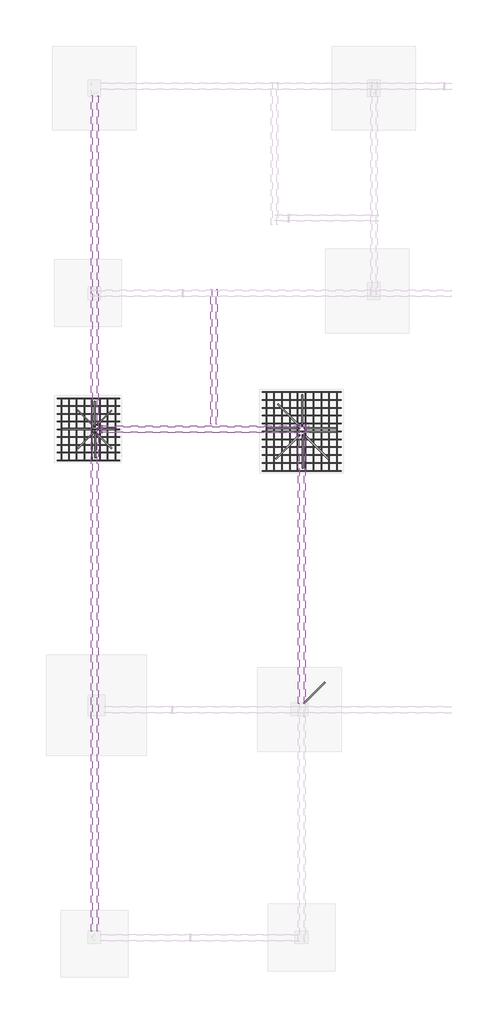
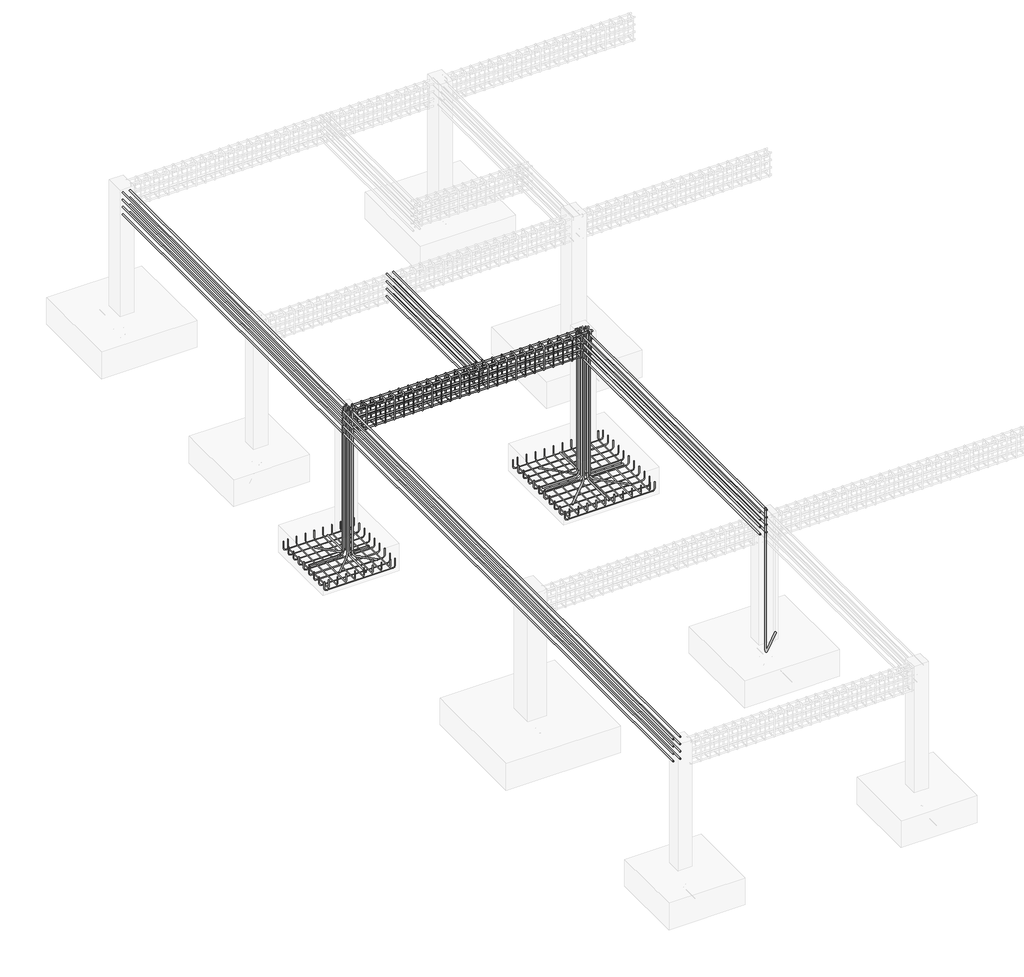
# One storey, part 5 of 10: 33 reinforcing bars.
"""IFC4 building model written with IfcOpenShell, lengths in millimetres."""

from ifc_helpers import new_model, si_unit, point, frame, origin, place, context, project, spatial, polyline, circle_curve, trimmed, segment, composite_curve, source, transform, mapped, element, save
from ifc_brep_helpers import swept_disk

model = new_model("IFC4")

# Units and contexts
model_context = context("Model", 3, world=origin())
ifc_project = project(units=[si_unit("LENGTHUNIT", "METRE", prefix="MILLI")], contexts=[model_context])

# Site, building, storey
site = spatial("IfcSite", under=ifc_project)
building = spatial("IfcBuilding", under=site)
storey = spatial("IfcBuildingStorey", under=building, Elevation=-2133.6)

# Reinforcing bars
placement = place(None, origin())
reinforcing_bar_shape = source(origin(), model_context, "Body", "SolidModel", [
    swept_disk(composite_curve([segment(polyline([(-4484.7164362, 6505.3219177, -2393.6), (-4484.7164362, 6505.3219177, -2504.1)]), True, "CONTINUOUS"), segment(trimmed(circle_curve(frame((-4519.4664362, 6505.3219177, -2504.1), z_axis=(0.0, 1.0, 0.0), x_axis=(34.75, 0.0, 0.0)), 34.75), [point((-4484.7164362, 6505.3219177, -2504.1))], [point((-4519.4664362, 6505.3219177, -2538.85))], True, "CARTESIAN"), True, "CONTINUOUS"), segment(polyline([(-4519.4664362, 6505.3219177, -2538.85), (-5579.6664362, 6505.3219177, -2538.85)]), True, "CONTINUOUS"), segment(trimmed(circle_curve(frame((-5579.6664362, 6505.3219177, -2504.1), z_axis=(0.0, 1.0, 0.0), x_axis=(0.0, 0.0, -34.75)), 34.75), [point((-5579.6664362, 6505.3219177, -2538.85))], [point((-5614.4164362, 6505.3219177, -2504.1))], True, "CARTESIAN"), True, "CONTINUOUS"), segment(polyline([(-5614.4164362, 6505.3219177, -2504.1), (-5614.4164362, 6505.3219177, -2393.6)]), True, "CONTINUOUS")], self_intersect=False), 4.75),
])
element("IfcReinforcingBar", 1, at=placement, inside=storey, context=model_context, shape_type="MappedRepresentation", body=[
    mapped(reinforcing_bar_shape, transform((0.0, 0.0, 0.0), x_axis=(1.0, 0.0, 0.0), y_axis=(0.0, 1.0, 0.0), z_axis=(0.0, 0.0, 1.0))),
    mapped(reinforcing_bar_shape, transform((0.0, -141.2125, 0.0), x_axis=(1.0, 0.0, 0.0), y_axis=(0.0, 1.0, 0.0), z_axis=(0.0, 0.0, 1.0))),
    mapped(reinforcing_bar_shape, transform((0.0, -282.425, 0.0), x_axis=(1.0, 0.0, 0.0), y_axis=(0.0, 1.0, 0.0), z_axis=(0.0, 0.0, 1.0))),
    mapped(reinforcing_bar_shape, transform((0.0, -423.6375, 0.0), x_axis=(1.0, 0.0, 0.0), y_axis=(0.0, 1.0, 0.0), z_axis=(0.0, 0.0, 1.0))),
    mapped(reinforcing_bar_shape, transform((0.0, -564.85, 0.0), x_axis=(1.0, 0.0, 0.0), y_axis=(0.0, 1.0, 0.0), z_axis=(0.0, 0.0, 1.0))),
    mapped(reinforcing_bar_shape, transform((0.0, -706.0625, 0.0), x_axis=(1.0, 0.0, 0.0), y_axis=(0.0, 1.0, 0.0), z_axis=(0.0, 0.0, 1.0))),
    mapped(reinforcing_bar_shape, transform((0.0, -847.275, 0.0), x_axis=(1.0, 0.0, 0.0), y_axis=(0.0, 1.0, 0.0), z_axis=(0.0, 0.0, 1.0))),
    mapped(reinforcing_bar_shape, transform((0.0, -988.4875, 0.0), x_axis=(1.0, 0.0, 0.0), y_axis=(0.0, 1.0, 0.0), z_axis=(0.0, 0.0, 1.0))),
    mapped(reinforcing_bar_shape, transform((0.0, -1129.7, 0.0), x_axis=(1.0, 0.0, 0.0), y_axis=(0.0, 1.0, 0.0), z_axis=(0.0, 0.0, 1.0))),
])
reinforcing_bar_2_shape = source(origin(), model_context, "Body", "SolidModel", [
    swept_disk(composite_curve([segment(polyline([(-4559.6743867, 5375.6219177, -2379.223371), (-4559.6743867, 5375.6219177, -2489.723371)]), True, "CONTINUOUS"), segment(trimmed(circle_curve(frame((-4559.6743867, 5410.3719177, -2489.723371), z_axis=(1.0, 0.0, 0.0), x_axis=(0.0, -34.75, 0.0)), 34.75), [point((-4559.6743867, 5375.6219177, -2489.723371))], [point((-4559.6743867, 5410.3719177, -2524.473371))], True, "CARTESIAN"), True, "CONTINUOUS"), segment(polyline([(-4559.6743867, 5410.3719177, -2524.473371), (-4559.6743867, 6470.5719177, -2524.473371)]), True, "CONTINUOUS"), segment(trimmed(circle_curve(frame((-4559.6743867, 6470.5719177, -2489.723371), z_axis=(1.0, 0.0, 0.0), x_axis=(0.0, 0.0, -34.75)), 34.75), [point((-4559.6743867, 6470.5719177, -2524.473371))], [point((-4559.6743867, 6505.3219177, -2489.723371))], True, "CARTESIAN"), True, "CONTINUOUS"), segment(polyline([(-4559.6743867, 6505.3219177, -2489.723371), (-4559.6743867, 6505.3219177, -2379.223371)]), True, "CONTINUOUS")], self_intersect=False), 4.75),
])
element("IfcReinforcingBar", 2, at=placement, inside=storey, context=model_context, shape_type="MappedRepresentation", body=[
    mapped(reinforcing_bar_2_shape, transform((0.0, 0.0, 0.0), x_axis=(1.0, 0.0, 0.0), y_axis=(0.0, 1.0, 0.0), z_axis=(0.0, 0.0, 1.0))),
    mapped(reinforcing_bar_2_shape, transform((-140.5079612, 0.0, 0.0), x_axis=(1.0, 0.0, 0.0), y_axis=(0.0, 1.0, 0.0), z_axis=(0.0, 0.0, 1.0))),
    mapped(reinforcing_bar_2_shape, transform((-281.0159224, 0.0, 0.0), x_axis=(1.0, 0.0, 0.0), y_axis=(0.0, 1.0, 0.0), z_axis=(0.0, 0.0, 1.0))),
    mapped(reinforcing_bar_2_shape, transform((-421.5238836, 0.0, 0.0), x_axis=(1.0, 0.0, 0.0), y_axis=(0.0, 1.0, 0.0), z_axis=(0.0, 0.0, 1.0))),
    mapped(reinforcing_bar_2_shape, transform((-562.0318448, 0.0, 0.0), x_axis=(1.0, 0.0, 0.0), y_axis=(0.0, 1.0, 0.0), z_axis=(0.0, 0.0, 1.0))),
    mapped(reinforcing_bar_2_shape, transform((-702.539806, 0.0, 0.0), x_axis=(1.0, 0.0, 0.0), y_axis=(0.0, 1.0, 0.0), z_axis=(0.0, 0.0, 1.0))),
    mapped(reinforcing_bar_2_shape, transform((-843.0477672, 0.0, 0.0), x_axis=(1.0, 0.0, 0.0), y_axis=(0.0, 1.0, 0.0), z_axis=(0.0, 0.0, 1.0))),
    mapped(reinforcing_bar_2_shape, transform((-983.5557284, 0.0, 0.0), x_axis=(1.0, 0.0, 0.0), y_axis=(0.0, 1.0, 0.0), z_axis=(0.0, 0.0, 1.0))),
])
reinforcing_bar_3_shape = source(origin(), model_context, "Body", "SolidModel", [
    swept_disk(composite_curve([segment(polyline([(-446.1164362, 6619.6219177, -2393.6), (-446.1164362, 6619.6219177, -2504.1)]), True, "CONTINUOUS"), segment(trimmed(circle_curve(frame((-480.8664362, 6619.6219177, -2504.1), z_axis=(0.0, 1.0, 0.0), x_axis=(34.75, 0.0, 0.0)), 34.75), [point((-446.1164362, 6619.6219177, -2504.1))], [point((-480.8664362, 6619.6219177, -2538.85))], True, "CARTESIAN"), True, "CONTINUOUS"), segment(polyline([(-480.8664362, 6619.6219177, -2538.85), (-1845.8664362, 6619.6219177, -2538.85)]), True, "CONTINUOUS"), segment(trimmed(circle_curve(frame((-1845.8664362, 6619.6219177, -2504.1), z_axis=(0.0, 1.0, 0.0), x_axis=(0.0, 0.0, -34.75)), 34.75), [point((-1845.8664362, 6619.6219177, -2538.85))], [point((-1880.6164362, 6619.6219177, -2504.1))], True, "CARTESIAN"), True, "CONTINUOUS"), segment(polyline([(-1880.6164362, 6619.6219177, -2504.1), (-1880.6164362, 6619.6219177, -2393.6)]), True, "CONTINUOUS")], self_intersect=False), 4.75),
])
element("IfcReinforcingBar", 3, at=placement, inside=storey, context=model_context, shape_type="MappedRepresentation", body=[
    mapped(reinforcing_bar_3_shape, transform((0.0, 0.0, 0.0), x_axis=(1.0, 0.0, 0.0), y_axis=(0.0, 1.0, 0.0), z_axis=(0.0, 0.0, 1.0))),
    mapped(reinforcing_bar_3_shape, transform((0.0, -143.45, 0.0), x_axis=(1.0, 0.0, 0.0), y_axis=(0.0, 1.0, 0.0), z_axis=(0.0, 0.0, 1.0))),
    mapped(reinforcing_bar_3_shape, transform((0.0, -286.9, 0.0), x_axis=(1.0, 0.0, 0.0), y_axis=(0.0, 1.0, 0.0), z_axis=(0.0, 0.0, 1.0))),
    mapped(reinforcing_bar_3_shape, transform((0.0, -430.35, 0.0), x_axis=(1.0, 0.0, 0.0), y_axis=(0.0, 1.0, 0.0), z_axis=(0.0, 0.0, 1.0))),
    mapped(reinforcing_bar_3_shape, transform((0.0, -573.8, 0.0), x_axis=(1.0, 0.0, 0.0), y_axis=(0.0, 1.0, 0.0), z_axis=(0.0, 0.0, 1.0))),
    mapped(reinforcing_bar_3_shape, transform((0.0, -717.25, 0.0), x_axis=(1.0, 0.0, 0.0), y_axis=(0.0, 1.0, 0.0), z_axis=(0.0, 0.0, 1.0))),
    mapped(reinforcing_bar_3_shape, transform((0.0, -860.7, 0.0), x_axis=(1.0, 0.0, 0.0), y_axis=(0.0, 1.0, 0.0), z_axis=(0.0, 0.0, 1.0))),
    mapped(reinforcing_bar_3_shape, transform((0.0, -1004.15, 0.0), x_axis=(1.0, 0.0, 0.0), y_axis=(0.0, 1.0, 0.0), z_axis=(0.0, 0.0, 1.0))),
    mapped(reinforcing_bar_3_shape, transform((0.0, -1147.6, 0.0), x_axis=(1.0, 0.0, 0.0), y_axis=(0.0, 1.0, 0.0), z_axis=(0.0, 0.0, 1.0))),
    mapped(reinforcing_bar_3_shape, transform((0.0, -1291.05, 0.0), x_axis=(1.0, 0.0, 0.0), y_axis=(0.0, 1.0, 0.0), z_axis=(0.0, 0.0, 1.0))),
    mapped(reinforcing_bar_3_shape, transform((0.0, -1434.5, 0.0), x_axis=(1.0, 0.0, 0.0), y_axis=(0.0, 1.0, 0.0), z_axis=(0.0, 0.0, 1.0))),
])
reinforcing_bar_4_shape = source(origin(), model_context, "Body", "SolidModel", [
    swept_disk(composite_curve([segment(polyline([(-521.0743867, 5185.1219177, -2379.223371), (-521.0743867, 5185.1219177, -2489.723371)]), True, "CONTINUOUS"), segment(trimmed(circle_curve(frame((-521.0743867, 5219.8719177, -2489.723371), z_axis=(1.0, 0.0, 0.0), x_axis=(0.0, -34.75, 0.0)), 34.75), [point((-521.0743867, 5185.1219177, -2489.723371))], [point((-521.0743867, 5219.8719177, -2524.473371))], True, "CARTESIAN"), True, "CONTINUOUS"), segment(polyline([(-521.0743867, 5219.8719177, -2524.473371), (-521.0743867, 6584.8719177, -2524.473371)]), True, "CONTINUOUS"), segment(trimmed(circle_curve(frame((-521.0743867, 6584.8719177, -2489.723371), z_axis=(1.0, 0.0, 0.0), x_axis=(0.0, 0.0, -34.75)), 34.75), [point((-521.0743867, 6584.8719177, -2524.473371))], [point((-521.0743867, 6619.6219177, -2489.723371))], True, "CARTESIAN"), True, "CONTINUOUS"), segment(polyline([(-521.0743867, 6619.6219177, -2489.723371), (-521.0743867, 6619.6219177, -2379.223371)]), True, "CONTINUOUS")], self_intersect=False), 4.75),
])
element("IfcReinforcingBar", 4, at=placement, inside=storey, context=model_context, shape_type="MappedRepresentation", body=[
    mapped(reinforcing_bar_4_shape, transform((0.0, 0.0, 0.0), x_axis=(1.0, 0.0, 0.0), y_axis=(0.0, 1.0, 0.0), z_axis=(0.0, 0.0, 1.0))),
    mapped(reinforcing_bar_4_shape, transform((-143.1506365, 0.0, 0.0), x_axis=(1.0, 0.0, 0.0), y_axis=(0.0, 1.0, 0.0), z_axis=(0.0, 0.0, 1.0))),
    mapped(reinforcing_bar_4_shape, transform((-286.301273, 0.0, 0.0), x_axis=(1.0, 0.0, 0.0), y_axis=(0.0, 1.0, 0.0), z_axis=(0.0, 0.0, 1.0))),
    mapped(reinforcing_bar_4_shape, transform((-429.4519095, 0.0, 0.0), x_axis=(1.0, 0.0, 0.0), y_axis=(0.0, 1.0, 0.0), z_axis=(0.0, 0.0, 1.0))),
    mapped(reinforcing_bar_4_shape, transform((-572.602546, 0.0, 0.0), x_axis=(1.0, 0.0, 0.0), y_axis=(0.0, 1.0, 0.0), z_axis=(0.0, 0.0, 1.0))),
    mapped(reinforcing_bar_4_shape, transform((-715.7531825, 0.0, 0.0), x_axis=(1.0, 0.0, 0.0), y_axis=(0.0, 1.0, 0.0), z_axis=(0.0, 0.0, 1.0))),
    mapped(reinforcing_bar_4_shape, transform((-858.903819, 0.0, 0.0), x_axis=(1.0, 0.0, 0.0), y_axis=(0.0, 1.0, 0.0), z_axis=(0.0, 0.0, 1.0))),
    mapped(reinforcing_bar_4_shape, transform((-1002.0544555, 0.0, 0.0), x_axis=(1.0, 0.0, 0.0), y_axis=(0.0, 1.0, 0.0), z_axis=(0.0, 0.0, 1.0))),
    mapped(reinforcing_bar_4_shape, transform((-1145.205092, 0.0, 0.0), x_axis=(1.0, 0.0, 0.0), y_axis=(0.0, 1.0, 0.0), z_axis=(0.0, 0.0, 1.0))),
    mapped(reinforcing_bar_4_shape, transform((-1288.3557284, 0.0, 0.0), x_axis=(1.0, 0.0, 0.0), y_axis=(0.0, 1.0, 0.0), z_axis=(0.0, 0.0, 1.0))),
])
element("IfcReinforcingBar", 5, at=placement, inside=storey, context=model_context, shape_type="SolidModel", body=[
    swept_disk(composite_curve([segment(polyline([(-4944.3664362, 5988.5552961, -40.0), (-4944.3664362, 5988.5552961, -2426.55)]), True, "CONTINUOUS"), segment(trimmed(circle_curve(frame((-4991.7779458, 6035.9668058, -2426.55), z_axis=(0.7071067811865519, 0.7071067811865431, 0.0), x_axis=(47.4115096000005, -47.41150969999944, 0.0)), 67.05), [point((-4944.3664362, 5988.5552961, -2426.55))], [point((-4991.7779458, 6035.9668058, -2493.6))], True, "CARTESIAN"), True, "CONTINUOUS"), segment(polyline([(-4991.7779458, 6035.9668058, -2493.6), (-5240.1883692, 6284.3772292, -2493.6)]), True, "CONTINUOUS")], self_intersect=False), 9.55),
])
element("IfcReinforcingBar", 6, at=placement, inside=storey, context=model_context, shape_type="SolidModel", body=[
    swept_disk(composite_curve([segment(polyline([(-4886.9664362, 6026.6552961, -40.0), (-4886.9664362, 6026.6552961, -2426.55)]), True, "CONTINUOUS"), segment(trimmed(circle_curve(frame((-4839.5549265, 6074.0668058, -2426.55), z_axis=(0.7071067811865519, -0.7071067811865431, 0.0), x_axis=(-47.41150970000035, -47.41150970000035, 0.0)), 67.05), [point((-4886.9664362, 6026.6552961, -2426.55))], [point((-4839.5549265, 6074.0668058, -2493.6))], True, "CARTESIAN"), True, "CONTINUOUS"), segment(polyline([(-4839.5549265, 6074.0668058, -2493.6), (-4629.2445031, 6284.3772292, -2493.6)]), True, "CONTINUOUS")], self_intersect=False), 9.55),
])
element("IfcReinforcingBar", 7, at=placement, inside=storey, context=model_context, shape_type="SolidModel", body=[
    swept_disk(composite_curve([segment(polyline([(-4944.3664362, 5892.3885393, -40.0), (-4944.3664362, 5892.3885393, -2426.55)]), True, "CONTINUOUS"), segment(trimmed(circle_curve(frame((-4991.7779458, 5844.9770296, -2426.55), z_axis=(-0.707106781186552, 0.7071067811865431, 0.0), x_axis=(47.4115096000005, 47.41150970000035, 0.0)), 67.05), [point((-4944.3664362, 5892.3885393, -2426.55))], [point((-4991.7779458, 5844.9770296, -2493.6))], True, "CARTESIAN"), True, "CONTINUOUS"), segment(polyline([(-4991.7779458, 5844.9770296, -2493.6), (-5240.1883692, 5596.5666062, -2493.6)]), True, "CONTINUOUS")], self_intersect=False), 9.55),
])
element("IfcReinforcingBar", 8, at=placement, inside=storey, context=model_context, shape_type="SolidModel", body=[
    swept_disk(composite_curve([segment(polyline([(-4886.9664362, 5854.2885393, -40.0), (-4886.9664362, 5854.2885393, -2426.55)]), True, "CONTINUOUS"), segment(trimmed(circle_curve(frame((-4839.5549265, 5806.8770296, -2426.55), z_axis=(-0.7071067811865519, -0.7071067811865431, 0.0), x_axis=(-47.41150970000035, 47.41150969999944, 0.0)), 67.05), [point((-4886.9664362, 5854.2885393, -2426.55))], [point((-4839.5549265, 5806.8770296, -2493.6))], True, "CARTESIAN"), True, "CONTINUOUS"), segment(polyline([(-4839.5549265, 5806.8770296, -2493.6), (-4629.2445031, 5596.5666062, -2493.6)]), True, "CONTINUOUS")], self_intersect=False), 9.55),
])
element("IfcReinforcingBar", 9, at=placement, inside=storey, context=model_context, shape_type="SolidModel", body=[
    swept_disk(composite_curve([segment(polyline([(-4933.5805145, 5988.5552961, -40.0), (-4933.5805145, 5988.5552961, -2426.55)]), True, "CONTINUOUS"), segment(trimmed(circle_curve(frame((-4933.5805145, 6055.6052961, -2426.55), z_axis=(1.0, 0.0, 0.0), x_axis=(0.0, -67.04999999999927, 0.0)), 67.05), [point((-4933.5805145, 5988.5552961, -2426.55))], [point((-4933.5805145, 6055.6052961, -2493.6))], True, "CARTESIAN"), True, "CONTINUOUS"), segment(polyline([(-4933.5805145, 6055.6052961, -2493.6), (-4933.5805145, 6454.2552961, -2493.6)]), True, "CONTINUOUS")], self_intersect=False), 9.55),
])
element("IfcReinforcingBar", 10, at=placement, inside=storey, context=model_context, shape_type="SolidModel", body=[
    swept_disk(composite_curve([segment(polyline([(-4923.5805145, 5892.3885393, -40.0), (-4923.5805145, 5892.3885393, -2426.55)]), True, "CONTINUOUS"), segment(trimmed(circle_curve(frame((-4923.5805145, 5825.3385393, -2426.55), z_axis=(-1.0, 0.0, 0.0), x_axis=(0.0, 67.05000000000018, 0.0)), 67.05), [point((-4923.5805145, 5892.3885393, -2426.55))], [point((-4923.5805145, 5825.3385393, -2493.6))], True, "CARTESIAN"), True, "CONTINUOUS"), segment(polyline([(-4923.5805145, 5825.3385393, -2493.6), (-4923.5805145, 5426.6885393, -2493.6)]), True, "CONTINUOUS")], self_intersect=False), 9.55),
])
element("IfcReinforcingBar", 11, at=placement, inside=storey, context=model_context, shape_type="SolidModel", body=[
    swept_disk(composite_curve([segment(polyline([(-4982.4664362, 5943.5552961, -40.0), (-4982.4664362, 5943.5552961, -2426.55)]), True, "CONTINUOUS"), segment(trimmed(circle_curve(frame((-5049.5164362, 5943.5552961, -2426.55), z_axis=(0.0, 1.0, 0.0), x_axis=(67.04999999999927, 0.0, 0.0)), 67.05), [point((-4982.4664362, 5943.5552961, -2426.55))], [point((-5049.5164362, 5943.5552961, -2493.6))], True, "CARTESIAN"), True, "CONTINUOUS"), segment(polyline([(-5049.5164362, 5943.5552961, -2493.6), (-5524.3664362, 5943.5552961, -2493.6)]), True, "CONTINUOUS")], self_intersect=False), 9.55),
])
element("IfcReinforcingBar", 12, at=placement, inside=storey, context=model_context, shape_type="SolidModel", body=[
    swept_disk(composite_curve([segment(polyline([(-4982.4664362, 5952.6170998, -40.0), (-4982.4664362, 5952.6170998, -2426.55)]), True, "CONTINUOUS"), segment(trimmed(circle_curve(frame((-5049.5164362, 5952.6170998, -2426.55), z_axis=(0.0, 1.0, 0.0), x_axis=(67.04999999999927, 0.0, 0.0)), 67.05), [point((-4982.4664362, 5952.6170998, -2426.55))], [point((-5049.5164362, 5952.6170998, -2493.6))], True, "CARTESIAN"), True, "CONTINUOUS"), segment(polyline([(-5049.5164362, 5952.6170998, -2493.6), (-5524.3664362, 5952.6170998, -2493.6)]), True, "CONTINUOUS")], self_intersect=False), 9.55),
])
element("IfcReinforcingBar", 13, at=placement, inside=storey, context=model_context, shape_type="SolidModel", body=[
    swept_disk(composite_curve([segment(polyline([(-4886.9664362, 5943.5552961, -40.0), (-4886.9664362, 5943.5552961, -2426.55)]), True, "CONTINUOUS"), segment(trimmed(circle_curve(frame((-4819.9164362, 5943.5552961, -2426.55), z_axis=(0.0, -1.0, 0.0), x_axis=(-67.05000000000018, 0.0, 0.0)), 67.05), [point((-4886.9664362, 5943.5552961, -2426.55))], [point((-4819.9164362, 5943.5552961, -2493.6))], True, "CARTESIAN"), True, "CONTINUOUS"), segment(polyline([(-4819.9164362, 5943.5552961, -2493.6), (-4573.6664362, 5943.5552961, -2493.6)]), True, "CONTINUOUS")], self_intersect=False), 9.55),
])
element("IfcReinforcingBar", 14, at=placement, inside=storey, context=model_context, shape_type="SolidModel", body=[
    swept_disk(composite_curve([segment(polyline([(-4886.9664362, 5952.6170998, -40.0), (-4886.9664362, 5952.6170998, -2426.55)]), True, "CONTINUOUS"), segment(trimmed(circle_curve(frame((-4819.9164362, 5952.6170998, -2426.55), z_axis=(0.0, -1.0, 0.0), x_axis=(-67.05000000000018, 0.0, 0.0)), 67.05), [point((-4886.9664362, 5952.6170998, -2426.55))], [point((-4819.9164362, 5952.6170998, -2493.6))], True, "CARTESIAN"), True, "CONTINUOUS"), segment(polyline([(-4819.9164362, 5952.6170998, -2493.6), (-4573.6664362, 5952.6170998, -2493.6)]), True, "CONTINUOUS")], self_intersect=False), 9.55),
])
element("IfcReinforcingBar", 15, at=placement, inside=storey, context=model_context, shape_type="SolidModel", body=[
    swept_disk(composite_curve([segment(polyline([(-1115.0664362, 959.3552961, -40.0), (-1115.0664362, 959.3552961, -2426.55)]), True, "CONTINUOUS"), segment(trimmed(circle_curve(frame((-1067.6549265, 1006.7668058, -2426.55), z_axis=(0.7071067811865519, -0.7071067811865431, 0.0), x_axis=(-47.4115096999999, -47.41150970000001, 0.0)), 67.05), [point((-1115.0664362, 959.3552961, -2426.55))], [point((-1067.6549265, 1006.7668058, -2493.6))], True, "CARTESIAN"), True, "CONTINUOUS"), segment(polyline([(-1067.6549265, 1006.7668058, -2493.6), (-743.0445031, 1331.3772292, -2493.6)]), True, "CONTINUOUS")], self_intersect=False), 9.55),
])
element("IfcReinforcingBar", 16, at=placement, inside=storey, context=model_context, shape_type="SolidModel", body=[
    swept_disk(composite_curve([segment(polyline([(-1205.4664362, 6006.6552961, -40.0), (-1205.4664362, 6006.6552961, -2426.55)]), True, "CONTINUOUS"), segment(trimmed(circle_curve(frame((-1252.8779458, 6054.0668058, -2426.55), z_axis=(0.7071067811865519, 0.7071067811865431, 0.0), x_axis=(47.41150959999982, -47.41150970000035, 0.0)), 67.05), [point((-1205.4664362, 6006.6552961, -2426.55))], [point((-1252.8779458, 6054.0668058, -2493.6))], True, "CARTESIAN"), True, "CONTINUOUS"), segment(polyline([(-1252.8779458, 6054.0668058, -2493.6), (-1597.4883692, 6398.6772292, -2493.6)]), True, "CONTINUOUS")], self_intersect=False), 9.55),
])
element("IfcReinforcingBar", 17, at=placement, inside=storey, context=model_context, shape_type="SolidModel", body=[
    swept_disk(composite_curve([segment(polyline([(-1205.4664362, 5834.2885393, -40.0), (-1205.4664362, 5834.2885393, -2426.55)]), True, "CONTINUOUS"), segment(trimmed(circle_curve(frame((-1252.8779458, 5786.8770296, -2426.55), z_axis=(-0.7071067811865519, 0.7071067811865431, 0.0), x_axis=(47.41150959999982, 47.41150969999944, 0.0)), 67.05), [point((-1205.4664362, 5834.2885393, -2426.55))], [point((-1252.8779458, 5786.8770296, -2493.6))], True, "CARTESIAN"), True, "CONTINUOUS"), segment(polyline([(-1252.8779458, 5786.8770296, -2493.6), (-1633.6883692, 5406.0666062, -2493.6)]), True, "CONTINUOUS")], self_intersect=False), 9.55),
])
element("IfcReinforcingBar", 18, at=placement, inside=storey, context=model_context, shape_type="SolidModel", body=[
    swept_disk(composite_curve([segment(polyline([(-1109.9664362, 5834.2885393, -40.0), (-1109.9664362, 5834.2885393, -2426.55)]), True, "CONTINUOUS"), segment(trimmed(circle_curve(frame((-1062.5549265, 5786.8770296, -2426.55), z_axis=(-0.7071067811865519, -0.7071067811865431, 0.0), x_axis=(-47.411509700000124, 47.41150969999944, 0.0)), 67.05), [point((-1109.9664362, 5834.2885393, -2426.55))], [point((-1062.5549265, 5786.8770296, -2493.6))], True, "CARTESIAN"), True, "CONTINUOUS"), segment(polyline([(-1062.5549265, 5786.8770296, -2493.6), (-681.7445031, 5406.0666062, -2493.6)]), True, "CONTINUOUS")], self_intersect=False), 9.55),
])
element("IfcReinforcingBar", 19, at=placement, inside=storey, context=model_context, shape_type="SolidModel", body=[
    swept_disk(composite_curve([segment(polyline([(-1156.5805145, 6006.6552961, -40.0), (-1156.5805145, 6006.6552961, -2426.55)]), True, "CONTINUOUS"), segment(trimmed(circle_curve(frame((-1156.5805145, 6073.7052961, -2426.55), z_axis=(1.0, 0.0, 0.0), x_axis=(0.0, -67.05000000000018, 0.0)), 67.05), [point((-1156.5805145, 6006.6552961, -2426.55))], [point((-1156.5805145, 6073.7052961, -2493.6))], True, "CARTESIAN"), True, "CONTINUOUS"), segment(polyline([(-1156.5805145, 6073.7052961, -2493.6), (-1156.5805145, 6568.5552961, -2493.6)]), True, "CONTINUOUS")], self_intersect=False), 9.55),
])
element("IfcReinforcingBar", 20, at=placement, inside=storey, context=model_context, shape_type="SolidModel", body=[
    swept_disk(composite_curve([segment(polyline([(-1146.5805145, 5834.2885393, -40.0), (-1146.5805145, 5834.2885393, -2426.55)]), True, "CONTINUOUS"), segment(trimmed(circle_curve(frame((-1146.5805145, 5767.2385393, -2426.55), z_axis=(-1.0, 0.0, 0.0), x_axis=(0.0, 67.04999999999927, 0.0)), 67.05), [point((-1146.5805145, 5834.2885393, -2426.55))], [point((-1146.5805145, 5767.2385393, -2493.6))], True, "CARTESIAN"), True, "CONTINUOUS"), segment(polyline([(-1146.5805145, 5767.2385393, -2493.6), (-1146.5805145, 5236.1885393, -2493.6)]), True, "CONTINUOUS")], self_intersect=False), 9.55),
])
element("IfcReinforcingBar", 21, at=placement, inside=storey, context=model_context, shape_type="SolidModel", body=[
    swept_disk(composite_curve([segment(polyline([(-1205.4664362, 5961.6552961, -40.0), (-1205.4664362, 5961.6552961, -2426.55)]), True, "CONTINUOUS"), segment(trimmed(circle_curve(frame((-1272.5164362, 5961.6552961, -2426.55), z_axis=(0.0, 1.0, 0.0), x_axis=(67.04999999999995, 0.0, 0.0)), 67.05), [point((-1205.4664362, 5961.6552961, -2426.55))], [point((-1272.5164362, 5961.6552961, -2493.6))], True, "CARTESIAN"), True, "CONTINUOUS"), segment(polyline([(-1272.5164362, 5961.6552961, -2493.6), (-1790.5664362, 5961.6552961, -2493.6)]), True, "CONTINUOUS")], self_intersect=False), 9.55),
])
element("IfcReinforcingBar", 22, at=placement, inside=storey, context=model_context, shape_type="SolidModel", body=[
    swept_disk(composite_curve([segment(polyline([(-1205.4664362, 5894.5170998, -40.0), (-1205.4664362, 5894.5170998, -2426.55)]), True, "CONTINUOUS"), segment(trimmed(circle_curve(frame((-1272.5164362, 5894.5170998, -2426.55), z_axis=(0.0, 1.0, 0.0), x_axis=(67.04999999999995, 0.0, 0.0)), 67.05), [point((-1205.4664362, 5894.5170998, -2426.55))], [point((-1272.5164362, 5894.5170998, -2493.6))], True, "CARTESIAN"), True, "CONTINUOUS"), segment(polyline([(-1272.5164362, 5894.5170998, -2493.6), (-1790.5664362, 5894.5170998, -2493.6)]), True, "CONTINUOUS")], self_intersect=False), 9.55),
])
element("IfcReinforcingBar", 23, at=placement, inside=storey, context=model_context, shape_type="SolidModel", body=[
    swept_disk(composite_curve([segment(polyline([(-1109.9664362, 5961.6552961, -40.0), (-1109.9664362, 5961.6552961, -2426.55)]), True, "CONTINUOUS"), segment(trimmed(circle_curve(frame((-1042.9164362, 5961.6552961, -2426.55), z_axis=(0.0, -1.0, 0.0), x_axis=(-67.05000000000018, 0.0, 0.0)), 67.05), [point((-1109.9664362, 5961.6552961, -2426.55))], [point((-1042.9164362, 5961.6552961, -2493.6))], True, "CARTESIAN"), True, "CONTINUOUS"), segment(polyline([(-1042.9164362, 5961.6552961, -2493.6), (-535.0664362, 5961.6552961, -2493.6)]), True, "CONTINUOUS")], self_intersect=False), 9.55),
])
element("IfcReinforcingBar", 24, at=placement, inside=storey, context=model_context, shape_type="SolidModel", body=[
    swept_disk(composite_curve([segment(polyline([(-1109.9664362, 5894.5170998, -40.0), (-1109.9664362, 5894.5170998, -2426.55)]), True, "CONTINUOUS"), segment(trimmed(circle_curve(frame((-1042.9164362, 5894.5170998, -2426.55), z_axis=(0.0, -1.0, 0.0), x_axis=(-67.05000000000018, 0.0, 0.0)), 67.05), [point((-1109.9664362, 5894.5170998, -2426.55))], [point((-1042.9164362, 5894.5170998, -2493.6))], True, "CARTESIAN"), True, "CONTINUOUS"), segment(polyline([(-1042.9164362, 5894.5170998, -2493.6), (-535.0664362, 5894.5170998, -2493.6)]), True, "CONTINUOUS")], self_intersect=False), 9.55),
])
reinforcing_bar_5_shape = source(origin(), model_context, "Body", "SolidModel", [
    swept_disk(composite_curve([segment(polyline([(-4990.0664362, 12024.7829308, -62.4471188), (-4990.0664362, -3200.8934989, -62.4471188)]), True, "CONTINUOUS")], self_intersect=False), 9.55),
])
element("IfcReinforcingBar", 25, at=placement, inside=storey, context=model_context, shape_type="MappedRepresentation", body=[
    mapped(reinforcing_bar_5_shape, transform((0.0, 0.0, 0.0), x_axis=(1.0, 0.0, 0.0), y_axis=(0.0, 1.0, 0.0), z_axis=(0.0, 0.0, 1.0))),
    mapped(reinforcing_bar_5_shape, transform((0.0, 0.0, -124.4315072), x_axis=(1.0, 0.0, 0.0), y_axis=(0.0, 1.0, 0.0), z_axis=(0.0, 0.0, 1.0))),
    mapped(reinforcing_bar_5_shape, transform((0.0, 0.0, -248.8630144), x_axis=(1.0, 0.0, 0.0), y_axis=(0.0, 1.0, 0.0), z_axis=(0.0, 0.0, 1.0))),
    mapped(reinforcing_bar_5_shape, transform((0.0, 0.0, -373.2945216), x_axis=(1.0, 0.0, 0.0), y_axis=(0.0, 1.0, 0.0), z_axis=(0.0, 0.0, 1.0))),
])
reinforcing_bar_6_shape = source(origin(), model_context, "Body", "SolidModel", [
    swept_disk(composite_curve([segment(polyline([(-4880.4664362, 12017.4755885, -62.4471188), (-4880.4664362, -3199.8489997, -62.4471188)]), True, "CONTINUOUS")], self_intersect=False), 9.55),
])
element("IfcReinforcingBar", 26, at=placement, inside=storey, context=model_context, shape_type="MappedRepresentation", body=[
    mapped(reinforcing_bar_6_shape, transform((0.0, 0.0, 0.0), x_axis=(1.0, 0.0, 0.0), y_axis=(0.0, 1.0, 0.0), z_axis=(0.0, 0.0, 1.0))),
    mapped(reinforcing_bar_6_shape, transform((0.0, 0.0, -124.4315072), x_axis=(1.0, 0.0, 0.0), y_axis=(0.0, 1.0, 0.0), z_axis=(0.0, 0.0, 1.0))),
    mapped(reinforcing_bar_6_shape, transform((0.0, 0.0, -248.8630144), x_axis=(1.0, 0.0, 0.0), y_axis=(0.0, 1.0, 0.0), z_axis=(0.0, 0.0, 1.0))),
    mapped(reinforcing_bar_6_shape, transform((0.0, 0.0, -373.2945216), x_axis=(1.0, 0.0, 0.0), y_axis=(0.0, 1.0, 0.0), z_axis=(0.0, 0.0, 1.0))),
])
reinforcing_bar_7_shape = source(origin(), model_context, "Body", "SolidModel", [
    swept_disk(composite_curve([segment(polyline([(-1215.555702, 6032.8719177, -62.1107341), (-1215.555702, 939.3065011, -62.1107341)]), True, "CONTINUOUS")], self_intersect=False), 9.55),
])
element("IfcReinforcingBar", 27, at=placement, inside=storey, context=model_context, shape_type="MappedRepresentation", body=[
    mapped(reinforcing_bar_7_shape, transform((0.0, 0.0, 0.0), x_axis=(1.0, 0.0, 0.0), y_axis=(0.0, 1.0, 0.0), z_axis=(0.0, 0.0, 1.0))),
    mapped(reinforcing_bar_7_shape, transform((0.0, 0.0, -125.2595106), x_axis=(1.0, 0.0, 0.0), y_axis=(0.0, 1.0, 0.0), z_axis=(0.0, 0.0, 1.0))),
    mapped(reinforcing_bar_7_shape, transform((0.0, 0.0, -250.5190212), x_axis=(1.0, 0.0, 0.0), y_axis=(0.0, 1.0, 0.0), z_axis=(0.0, 0.0, 1.0))),
    mapped(reinforcing_bar_7_shape, transform((0.0, 0.0, -375.7785317), x_axis=(1.0, 0.0, 0.0), y_axis=(0.0, 1.0, 0.0), z_axis=(0.0, 0.0, 1.0))),
])
reinforcing_bar_8_shape = source(origin(), model_context, "Body", "SolidModel", [
    swept_disk(composite_curve([segment(polyline([(-1111.1771703, 6032.8719177, -62.1107341), (-1111.1771703, 940.3510003, -62.1107341)]), True, "CONTINUOUS")], self_intersect=False), 9.55),
])
element("IfcReinforcingBar", 28, at=placement, inside=storey, context=model_context, shape_type="MappedRepresentation", body=[
    mapped(reinforcing_bar_8_shape, transform((0.0, 0.0, 0.0), x_axis=(1.0, 0.0, 0.0), y_axis=(0.0, 1.0, 0.0), z_axis=(0.0, 0.0, 1.0))),
    mapped(reinforcing_bar_8_shape, transform((0.0, 0.0, -125.2595106), x_axis=(1.0, 0.0, 0.0), y_axis=(0.0, 1.0, 0.0), z_axis=(0.0, 0.0, 1.0))),
    mapped(reinforcing_bar_8_shape, transform((0.0, 0.0, -250.5190212), x_axis=(1.0, 0.0, 0.0), y_axis=(0.0, 1.0, 0.0), z_axis=(0.0, 0.0, 1.0))),
    mapped(reinforcing_bar_8_shape, transform((0.0, 0.0, -375.7785317), x_axis=(1.0, 0.0, 0.0), y_axis=(0.0, 1.0, 0.0), z_axis=(0.0, 0.0, 1.0))),
])
reinforcing_bar_9_shape = source(origin(), model_context, "Body", "SolidModel", [
    swept_disk(composite_curve([segment(polyline([(-4798.5997388, 5970.5786993, -109.4049959), (-4798.5997388, 5913.1728105, -51.9991072)]), True, "CONTINUOUS"), segment(trimmed(circle_curve(frame((-4798.5997388, 5895.6719177, -69.5), z_axis=(1.0, 0.0, 0.0), x_axis=(0.0, 17.500892799999747, 17.500892800000003)), 24.75), [point((-4798.5997388, 5913.1728105, -51.9991072))], [point((-4798.5997388, 5870.9219177, -69.5))], True, "CARTESIAN"), True, "CONTINUOUS"), segment(polyline([(-4798.5997388, 5870.9219177, -69.5), (-4798.5997388, 5870.9219177, -430.5)]), True, "CONTINUOUS"), segment(trimmed(circle_curve(frame((-4798.5997388, 5895.6719177, -430.5), z_axis=(1.0, 0.0, 0.0), x_axis=(0.0, -24.75, 0.0)), 24.75), [point((-4798.5997388, 5870.9219177, -430.5))], [point((-4798.5997388, 5895.6719177, -455.25))], True, "CARTESIAN"), True, "CONTINUOUS"), segment(polyline([(-4798.5997388, 5895.6719177, -455.25), (-4798.5997388, 5985.2719177, -455.25)]), True, "CONTINUOUS"), segment(trimmed(circle_curve(frame((-4799.1723626, 5985.2719177, -430.5066251), z_axis=(0.9997323196529888, 0.0, 0.02313631434032496), x_axis=(0.572623800000656, 0.0, -24.743374899999992)), 24.75), [point((-4798.5997388, 5985.2719177, -455.25))], [point((-4799.1723626, 6010.0219177, -430.5066251))], True, "CARTESIAN"), True, "CONTINUOUS"), segment(polyline([(-4799.1723626, 6010.0219177, -430.5066251), (-4807.527115, 6010.0219177, -69.4933749)]), True, "CONTINUOUS"), segment(trimmed(circle_curve(frame((-4807.527115, 5985.2719177, -69.4933749), z_axis=(0.9997323196529888, 0.0, 0.02313631434032496), x_axis=(0.0, 24.75, 0.0)), 24.75), [point((-4807.527115, 6010.0219177, -69.4933749))], [point((-4808.0997388, 5985.2719177, -44.75))], True, "CARTESIAN"), True, "CONTINUOUS"), segment(polyline([(-4808.0997388, 5985.2719177, -44.75), (-4808.0997388, 5895.6719177, -44.75)]), True, "CONTINUOUS"), segment(trimmed(circle_curve(frame((-4808.0997388, 5895.6719177, -69.5), z_axis=(1.0, 0.0, 0.0), x_axis=(0.0, 0.0, 24.75)), 24.75), [point((-4808.0997388, 5895.6719177, -44.75))], [point((-4808.0997388, 5878.1710249, -87.0008928))], True, "CARTESIAN"), True, "CONTINUOUS"), segment(polyline([(-4808.0997388, 5878.1710249, -87.0008928), (-4808.0997388, 5935.5769136, -144.4067815)]), True, "CONTINUOUS")], self_intersect=False), 4.75),
])
element("IfcReinforcingBar", 29, at=placement, inside=storey, context=model_context, shape_type="MappedRepresentation", body=[
    mapped(reinforcing_bar_9_shape, transform((0.0, 0.0, 0.0), x_axis=(1.0, 0.0, 0.0), y_axis=(0.0, 1.0, 0.0), z_axis=(0.0, 0.0, 1.0))),
    mapped(reinforcing_bar_9_shape, transform((149.2405569, 0.0, 0.0), x_axis=(1.0, 0.0, 0.0), y_axis=(0.0, 1.0, 0.0), z_axis=(0.0, 0.0, 1.0))),
    mapped(reinforcing_bar_9_shape, transform((298.4811139, 0.0, 0.0), x_axis=(1.0, 0.0, 0.0), y_axis=(0.0, 1.0, 0.0), z_axis=(0.0, 0.0, 1.0))),
    mapped(reinforcing_bar_9_shape, transform((447.7216708, 0.0, 0.0), x_axis=(1.0, 0.0, 0.0), y_axis=(0.0, 1.0, 0.0), z_axis=(0.0, 0.0, 1.0))),
    mapped(reinforcing_bar_9_shape, transform((596.9622277, 0.0, 0.0), x_axis=(1.0, 0.0, 0.0), y_axis=(0.0, 1.0, 0.0), z_axis=(0.0, 0.0, 1.0))),
    mapped(reinforcing_bar_9_shape, transform((746.2027846, 0.0, 0.0), x_axis=(1.0, 0.0, 0.0), y_axis=(0.0, 1.0, 0.0), z_axis=(0.0, 0.0, 1.0))),
    mapped(reinforcing_bar_9_shape, transform((895.4433416, 0.0, 0.0), x_axis=(1.0, 0.0, 0.0), y_axis=(0.0, 1.0, 0.0), z_axis=(0.0, 0.0, 1.0))),
    mapped(reinforcing_bar_9_shape, transform((1044.6838985, 0.0, 0.0), x_axis=(1.0, 0.0, 0.0), y_axis=(0.0, 1.0, 0.0), z_axis=(0.0, 0.0, 1.0))),
    mapped(reinforcing_bar_9_shape, transform((1193.9244554, 0.0, 0.0), x_axis=(1.0, 0.0, 0.0), y_axis=(0.0, 1.0, 0.0), z_axis=(0.0, 0.0, 1.0))),
    mapped(reinforcing_bar_9_shape, transform((1343.1650124, 0.0, 0.0), x_axis=(1.0, 0.0, 0.0), y_axis=(0.0, 1.0, 0.0), z_axis=(0.0, 0.0, 1.0))),
    mapped(reinforcing_bar_9_shape, transform((1492.4055693, 0.0, 0.0), x_axis=(1.0, 0.0, 0.0), y_axis=(0.0, 1.0, 0.0), z_axis=(0.0, 0.0, 1.0))),
    mapped(reinforcing_bar_9_shape, transform((1641.6461262, 0.0, 0.0), x_axis=(1.0, 0.0, 0.0), y_axis=(0.0, 1.0, 0.0), z_axis=(0.0, 0.0, 1.0))),
    mapped(reinforcing_bar_9_shape, transform((1790.8866831, 0.0, 0.0), x_axis=(1.0, 0.0, 0.0), y_axis=(0.0, 1.0, 0.0), z_axis=(0.0, 0.0, 1.0))),
    mapped(reinforcing_bar_9_shape, transform((1940.1272401, 0.0, 0.0), x_axis=(1.0, 0.0, 0.0), y_axis=(0.0, 1.0, 0.0), z_axis=(0.0, 0.0, 1.0))),
    mapped(reinforcing_bar_9_shape, transform((2089.367797, 0.0, 0.0), x_axis=(1.0, 0.0, 0.0), y_axis=(0.0, 1.0, 0.0), z_axis=(0.0, 0.0, 1.0))),
    mapped(reinforcing_bar_9_shape, transform((2238.6083539, 0.0, 0.0), x_axis=(1.0, 0.0, 0.0), y_axis=(0.0, 1.0, 0.0), z_axis=(0.0, 0.0, 1.0))),
    mapped(reinforcing_bar_9_shape, transform((2387.8489108, 0.0, 0.0), x_axis=(1.0, 0.0, 0.0), y_axis=(0.0, 1.0, 0.0), z_axis=(0.0, 0.0, 1.0))),
    mapped(reinforcing_bar_9_shape, transform((2537.0894678, 0.0, 0.0), x_axis=(1.0, 0.0, 0.0), y_axis=(0.0, 1.0, 0.0), z_axis=(0.0, 0.0, 1.0))),
    mapped(reinforcing_bar_9_shape, transform((2686.3300247, 0.0, 0.0), x_axis=(1.0, 0.0, 0.0), y_axis=(0.0, 1.0, 0.0), z_axis=(0.0, 0.0, 1.0))),
    mapped(reinforcing_bar_9_shape, transform((2835.5705816, 0.0, 0.0), x_axis=(1.0, 0.0, 0.0), y_axis=(0.0, 1.0, 0.0), z_axis=(0.0, 0.0, 1.0))),
    mapped(reinforcing_bar_9_shape, transform((2984.8111386, 0.0, 0.0), x_axis=(1.0, 0.0, 0.0), y_axis=(0.0, 1.0, 0.0), z_axis=(0.0, 0.0, 1.0))),
    mapped(reinforcing_bar_9_shape, transform((3134.0516955, 0.0, 0.0), x_axis=(1.0, 0.0, 0.0), y_axis=(0.0, 1.0, 0.0), z_axis=(0.0, 0.0, 1.0))),
    mapped(reinforcing_bar_9_shape, transform((3283.2922524, 0.0, 0.0), x_axis=(1.0, 0.0, 0.0), y_axis=(0.0, 1.0, 0.0), z_axis=(0.0, 0.0, 1.0))),
    mapped(reinforcing_bar_9_shape, transform((3432.5328093, 0.0, 0.0), x_axis=(1.0, 0.0, 0.0), y_axis=(0.0, 1.0, 0.0), z_axis=(0.0, 0.0, 1.0))),
    mapped(reinforcing_bar_9_shape, transform((3581.7733663, 0.0, 0.0), x_axis=(1.0, 0.0, 0.0), y_axis=(0.0, 1.0, 0.0), z_axis=(0.0, 0.0, 1.0))),
    mapped(reinforcing_bar_9_shape, transform((3731.0139232, 0.0, 0.0), x_axis=(1.0, 0.0, 0.0), y_axis=(0.0, 1.0, 0.0), z_axis=(0.0, 0.0, 1.0))),
])
reinforcing_bar_10_shape = source(origin(), model_context, "Body", "SolidModel", [
    swept_disk(composite_curve([segment(polyline([(-4824.2022232, 5888.2826519, -62.1107341), (-1033.9010196, 5888.2826519, -62.1107341)]), True, "CONTINUOUS")], self_intersect=False), 9.55),
])
element("IfcReinforcingBar", 30, at=placement, inside=storey, context=model_context, shape_type="MappedRepresentation", body=[
    mapped(reinforcing_bar_10_shape, transform((0.0, 0.0, 0.0), x_axis=(1.0, 0.0, 0.0), y_axis=(0.0, 1.0, 0.0), z_axis=(0.0, 0.0, 1.0))),
    mapped(reinforcing_bar_10_shape, transform((0.0, 0.0, -125.2595106), x_axis=(1.0, 0.0, 0.0), y_axis=(0.0, 1.0, 0.0), z_axis=(0.0, 0.0, 1.0))),
    mapped(reinforcing_bar_10_shape, transform((0.0, 0.0, -250.5190212), x_axis=(1.0, 0.0, 0.0), y_axis=(0.0, 1.0, 0.0), z_axis=(0.0, 0.0, 1.0))),
    mapped(reinforcing_bar_10_shape, transform((0.0, 0.0, -375.7785317), x_axis=(1.0, 0.0, 0.0), y_axis=(0.0, 1.0, 0.0), z_axis=(0.0, 0.0, 1.0))),
])
reinforcing_bar_11_shape = source(origin(), model_context, "Body", "SolidModel", [
    swept_disk(composite_curve([segment(polyline([(-4822.0555576, 5992.6611836, -62.1107341), (-1034.9455187, 5992.6611836, -62.1107341)]), True, "CONTINUOUS")], self_intersect=False), 9.55),
])
element("IfcReinforcingBar", 31, at=placement, inside=storey, context=model_context, shape_type="MappedRepresentation", body=[
    mapped(reinforcing_bar_11_shape, transform((0.0, 0.0, 0.0), x_axis=(1.0, 0.0, 0.0), y_axis=(0.0, 1.0, 0.0), z_axis=(0.0, 0.0, 1.0))),
    mapped(reinforcing_bar_11_shape, transform((0.0, 0.0, -125.2595106), x_axis=(1.0, 0.0, 0.0), y_axis=(0.0, 1.0, 0.0), z_axis=(0.0, 0.0, 1.0))),
    mapped(reinforcing_bar_11_shape, transform((0.0, 0.0, -250.5190212), x_axis=(1.0, 0.0, 0.0), y_axis=(0.0, 1.0, 0.0), z_axis=(0.0, 0.0, 1.0))),
    mapped(reinforcing_bar_11_shape, transform((0.0, 0.0, -375.7785317), x_axis=(1.0, 0.0, 0.0), y_axis=(0.0, 1.0, 0.0), z_axis=(0.0, 0.0, 1.0))),
])
reinforcing_bar_12_shape = source(origin(), model_context, "Body", "SolidModel", [
    swept_disk(composite_curve([segment(polyline([(-2815.755702, 8491.2719177, -62.1107341), (-2815.755702, 6034.982619, -62.1107341)]), True, "CONTINUOUS")], self_intersect=False), 9.55),
])
element("IfcReinforcingBar", 32, at=placement, inside=storey, context=model_context, shape_type="MappedRepresentation", body=[
    mapped(reinforcing_bar_12_shape, transform((0.0, 0.0, 0.0), x_axis=(1.0, 0.0, 0.0), y_axis=(0.0, 1.0, 0.0), z_axis=(0.0, 0.0, 1.0))),
    mapped(reinforcing_bar_12_shape, transform((0.0, 0.0, -125.2595106), x_axis=(1.0, 0.0, 0.0), y_axis=(0.0, 1.0, 0.0), z_axis=(0.0, 0.0, 1.0))),
    mapped(reinforcing_bar_12_shape, transform((0.0, 0.0, -250.5190212), x_axis=(1.0, 0.0, 0.0), y_axis=(0.0, 1.0, 0.0), z_axis=(0.0, 0.0, 1.0))),
    mapped(reinforcing_bar_12_shape, transform((0.0, 0.0, -375.7785317), x_axis=(1.0, 0.0, 0.0), y_axis=(0.0, 1.0, 0.0), z_axis=(0.0, 0.0, 1.0))),
])
reinforcing_bar_13_shape = source(origin(), model_context, "Body", "SolidModel", [
    swept_disk(composite_curve([segment(polyline([(-2711.3771703, 8491.2719177, -62.1107341), (-2711.3771703, 6031.0112374, -62.1107341)]), True, "CONTINUOUS")], self_intersect=False), 9.55),
])
element("IfcReinforcingBar", 33, at=placement, inside=storey, context=model_context, shape_type="MappedRepresentation", body=[
    mapped(reinforcing_bar_13_shape, transform((0.0, 0.0, 0.0), x_axis=(1.0, 0.0, 0.0), y_axis=(0.0, 1.0, 0.0), z_axis=(0.0, 0.0, 1.0))),
    mapped(reinforcing_bar_13_shape, transform((0.0, 0.0, -125.2595106), x_axis=(1.0, 0.0, 0.0), y_axis=(0.0, 1.0, 0.0), z_axis=(0.0, 0.0, 1.0))),
    mapped(reinforcing_bar_13_shape, transform((0.0, 0.0, -250.5190212), x_axis=(1.0, 0.0, 0.0), y_axis=(0.0, 1.0, 0.0), z_axis=(0.0, 0.0, 1.0))),
    mapped(reinforcing_bar_13_shape, transform((0.0, 0.0, -375.7785317), x_axis=(1.0, 0.0, 0.0), y_axis=(0.0, 1.0, 0.0), z_axis=(0.0, 0.0, 1.0))),
])

save(model, "model.ifc")

# Revit data of these elements
# Elements 1, 2, 3, 4, 5, 6, 7, 8, 9, 10, 11, 12, 13, 14, 15, 16, 17, 18, 19, 20, 21, 22, 23, 24, 25, 26, 27, 28, 29, 30, 31, 32, 33 (IfcReinforcingBar)
#   Phase Created = New Construction
